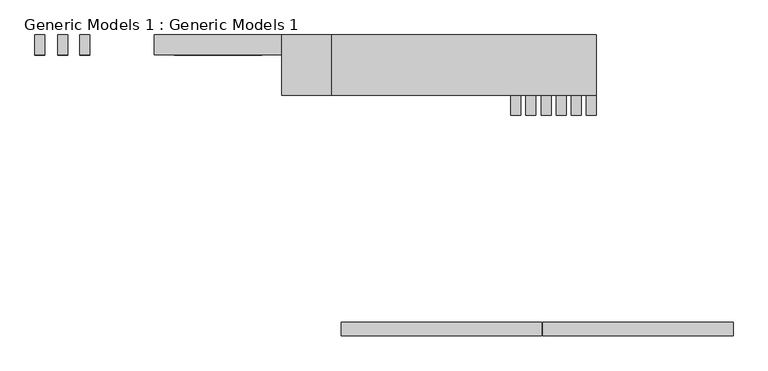
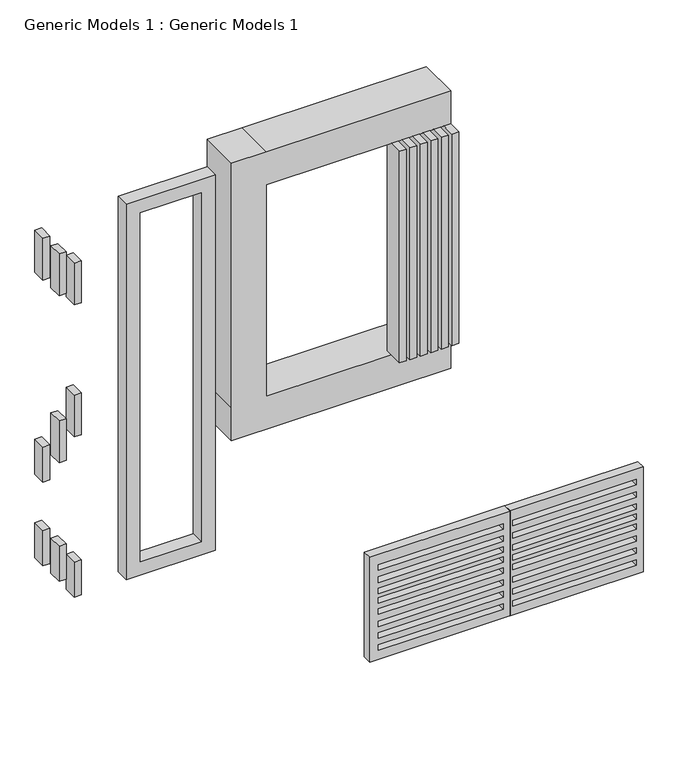
"""IFC4 building model written with IfcOpenShell, lengths in millimetres: proxy geometry, Generic Models 1 : Generic Models 1."""

from ifc_helpers import new_model, si_unit, frame, origin, place, context, project, spatial, polyline, outline, extrude, source, transform, mapped, element, save


def generic_models_1_generic_models_1_2996b52b(model_context):
    return source(origin(), model_context, "Body", "SweptSolid", [
        extrude(outline(polyline([(2263.7323709, 2503.9584916), (-152.4, 2503.9584916), (-152.4, 5399.5584916), (2263.7323709, 5399.5584916), (2263.7323709, 2503.9584916)]), holes=[polyline([(1900.2353757, 2559.0491365), (2027.2353757, 2559.0491365), (2027.2353757, 5251.4491365), (1900.2353757, 5251.4491365), (1900.2353757, 2559.0491365)]), polyline([(1620.8353757, 2559.0491365), (1747.8353757, 2559.0491365), (1747.8353757, 5251.4491365), (1620.8353757, 5251.4491365), (1620.8353757, 2559.0491365)]), polyline([(1341.4353757, 2559.0491365), (1468.4353757, 2559.0491365), (1468.4353757, 5251.4491365), (1341.4353757, 5251.4491365), (1341.4353757, 2559.0491365)]), polyline([(1112.8353757, 2559.0491365), (1239.8353757, 2559.0491365), (1239.8353757, 5251.4491365), (1112.8353757, 5251.4491365), (1112.8353757, 2559.0491365)]), polyline([(884.2353757, 2559.0491365), (1011.2353757, 2559.0491365), (1011.2353757, 5251.4491365), (884.2353757, 5251.4491365), (884.2353757, 2559.0491365)]), polyline([(604.8353757, 2559.0491365), (731.8353757, 2559.0491365), (731.8353757, 5251.4491365), (604.8353757, 5251.4491365), (604.8353757, 2559.0491365)]), polyline([(325.4353757, 2559.0491365), (452.4353757, 2559.0491365), (452.4353757, 5251.4491365), (325.4353757, 5251.4491365), (325.4353757, 2559.0491365)]), polyline([(46.0353757, 2559.0491365), (173.0353757, 2559.0491365), (173.0353757, 5251.4491365), (46.0353757, 5251.4491365), (46.0353757, 2559.0491365)])]), frame((0.0, -10129.8064015, 0.0), z_axis=(0.0, 1.0, 0.0), x_axis=(0.0, 0.0, 1.0)), (0.0, 0.0, 1.0), 203.2),
        extrude(outline(polyline([(-152.4, 2491.2584916), (2263.7323709, 2491.2584916), (2263.7323709, -556.7415084), (-152.4, -556.7415084), (-152.4, 2491.2584916)]), holes=[polyline([(1900.2353757, -369.7660375), (2027.2353757, -369.7660375), (2027.2353757, 2348.0339625), (1900.2353757, 2348.0339625), (1900.2353757, -369.7660375)]), polyline([(1620.8353757, -369.7660375), (1747.8353757, -369.7660375), (1747.8353757, 2348.0339625), (1620.8353757, 2348.0339625), (1620.8353757, -369.7660375)]), polyline([(1366.8353757, -369.7660375), (1493.8353757, -369.7660375), (1493.8353757, 2348.0339625), (1366.8353757, 2348.0339625), (1366.8353757, -369.7660375)]), polyline([(1138.2353757, -369.7660375), (1265.2353757, -369.7660375), (1265.2353757, 2348.0339625), (1138.2353757, 2348.0339625), (1138.2353757, -369.7660375)]), polyline([(884.2353757, -369.7660375), (1011.2353757, -369.7660375), (1011.2353757, 2348.0339625), (884.2353757, 2348.0339625), (884.2353757, -369.7660375)]), polyline([(604.8353757, -369.7660375), (731.8353757, -369.7660375), (731.8353757, 2348.0339625), (604.8353757, 2348.0339625), (604.8353757, -369.7660375)]), polyline([(335.2131579, -369.7660375), (462.2131579, -369.7660375), (462.2131579, 2348.0339625), (335.2131579, 2348.0339625), (335.2131579, -369.7660375)]), polyline([(55.8131579, -369.7660375), (182.8131579, -369.7660375), (182.8131579, 2348.0339625), (55.8131579, 2348.0339625), (55.8131579, -369.7660375)])]), frame((0.0, -10129.8064015, 0.0), z_axis=(0.0, 1.0, 0.0), x_axis=(0.0, 0.0, 1.0)), (0.0, 0.0, 1.0), 203.2),
        extrude(outline(polyline([(-5065.2415084, -5862.6064015), (-5217.6415084, -5862.6064015), (-5217.6415084, -5557.8064015), (-5065.2415084, -5557.8064015), (-5065.2415084, -5862.6064015)])), frame((0.0, 0.0, 7700.2105263), z_axis=(0.0, 0.0, 1.0), x_axis=(1.0, 0.0, 0.0)), (0.0, 0.0, 1.0), 962.5263158),
        extrude(outline(polyline([(-4715.583357, -5862.6064015), (-4867.983357, -5862.6064015), (-4867.983357, -5557.8064015), (-4715.583357, -5557.8064015), (-4715.583357, -5862.6064015)])), frame((0.0, 0.0, 7218.9473684), z_axis=(0.0, 0.0, 1.0), x_axis=(1.0, 0.0, 0.0)), (0.0, 0.0, 1.0), 962.5263158),
        extrude(outline(polyline([(-4386.7201991, -5862.6064015), (-4539.1201991, -5862.6064015), (-4539.1201991, -5557.8064015), (-4386.7201991, -5557.8064015), (-4386.7201991, -5862.6064015)])), frame((0.0, 0.0, 6890.0842105), z_axis=(0.0, 0.0, 1.0), x_axis=(1.0, 0.0, 0.0)), (0.0, 0.0, 1.0), 962.5263158),
        extrude(outline(polyline([(-5065.2415084, -5862.6064015), (-5217.6415084, -5862.6064015), (-5217.6415084, -5557.8064015), (-5065.2415084, -5557.8064015), (-5065.2415084, -5862.6064015)])), frame((0.0, 0.0, 3039.9789474), z_axis=(0.0, 0.0, 1.0), x_axis=(1.0, 0.0, 0.0)), (0.0, 0.0, 1.0), 810.1263158),
        extrude(outline(polyline([(-4715.583357, -5862.6064015), (-4867.983357, -5862.6064015), (-4867.983357, -5557.8064015), (-4715.583357, -5557.8064015), (-4715.583357, -5862.6064015)])), frame((0.0, 0.0, 3368.8421053), z_axis=(0.0, 0.0, 1.0), x_axis=(1.0, 0.0, 0.0)), (0.0, 0.0, 1.0), 962.5263158),
        extrude(outline(polyline([(-4386.7201991, -5862.6064015), (-4539.1201991, -5862.6064015), (-4539.1201991, -5557.8064015), (-4386.7201991, -5557.8064015), (-4386.7201991, -5862.6064015)])), frame((0.0, 0.0, 3850.1052632), z_axis=(0.0, 0.0, 1.0), x_axis=(1.0, 0.0, 0.0)), (0.0, 0.0, 1.0), 962.5263158),
        extrude(outline(polyline([(-5065.2415084, -5862.6064015), (-5217.6415084, -5862.6064015), (-5217.6415084, -5557.8064015), (-5065.2415084, -5557.8064015), (-5065.2415084, -5862.6064015)])), frame((0.0, 0.0, 1114.9263158), z_axis=(0.0, 0.0, 1.0), x_axis=(1.0, 0.0, 0.0)), (0.0, 0.0, 1.0), 810.1263158),
        extrude(outline(polyline([(-4715.583357, -5862.6064015), (-4867.983357, -5862.6064015), (-4867.983357, -5557.8064015), (-4715.583357, -5557.8064015), (-4715.583357, -5862.6064015)])), frame((0.0, 0.0, 633.6631579), z_axis=(0.0, 0.0, 1.0), x_axis=(1.0, 0.0, 0.0)), (0.0, 0.0, 1.0), 810.1263158),
        extrude(outline(polyline([(-4386.7201991, -5862.6064015), (-4539.1201991, -5862.6064015), (-4539.1201991, -5557.8064015), (-4386.7201991, -5557.8064015), (-4386.7201991, -5862.6064015)])), frame((0.0, 0.0, 152.4), z_axis=(0.0, 0.0, 1.0), x_axis=(1.0, 0.0, 0.0)), (0.0, 0.0, 1.0), 810.1263158),
        extrude(outline(polyline([(3316.7584916, -6777.0064015), (3164.3584916, -6777.0064015), (3164.3584916, -6319.8064015), (3316.7584916, -6319.8064015), (3316.7584916, -6777.0064015)])), frame((0.0, 0.0, 3810.0), z_axis=(0.0, 0.0, 1.0), x_axis=(1.0, 0.0, 0.0)), (0.0, 0.0, 1.0), 4876.8),
        extrude(outline(polyline([(3088.1584916, -6777.0064015), (2935.7584916, -6777.0064015), (2935.7584916, -6319.8064015), (3088.1584916, -6319.8064015), (3088.1584916, -6777.0064015)])), frame((0.0, 0.0, 3810.0), z_axis=(0.0, 0.0, 1.0), x_axis=(1.0, 0.0, 0.0)), (0.0, 0.0, 1.0), 4876.8),
        extrude(outline(polyline([(2859.5584916, -6777.0064015), (2707.1584916, -6777.0064015), (2707.1584916, -6319.8064015), (2859.5584916, -6319.8064015), (2859.5584916, -6777.0064015)])), frame((0.0, 0.0, 3810.0), z_axis=(0.0, 0.0, 1.0), x_axis=(1.0, 0.0, 0.0)), (0.0, 0.0, 1.0), 4876.8),
        extrude(outline(polyline([(2630.9584916, -6777.0064015), (2478.5584916, -6777.0064015), (2478.5584916, -6319.8064015), (2630.9584916, -6319.8064015), (2630.9584916, -6777.0064015)])), frame((0.0, 0.0, 3810.0), z_axis=(0.0, 0.0, 1.0), x_axis=(1.0, 0.0, 0.0)), (0.0, 0.0, 1.0), 4876.8),
        extrude(outline(polyline([(2402.3584916, -6777.0064015), (2249.9584916, -6777.0064015), (2249.9584916, -6319.8064015), (2402.3584916, -6319.8064015), (2402.3584916, -6777.0064015)])), frame((0.0, 0.0, 3810.0), z_axis=(0.0, 0.0, 1.0), x_axis=(1.0, 0.0, 0.0)), (0.0, 0.0, 1.0), 4876.8),
        extrude(outline(polyline([(2173.7584916, -6777.0064015), (2021.3584916, -6777.0064015), (2021.3584916, -6319.8064015), (2173.7584916, -6319.8064015), (2173.7584916, -6777.0064015)])), frame((0.0, 0.0, 3810.0), z_axis=(0.0, 0.0, 1.0), x_axis=(1.0, 0.0, 0.0)), (0.0, 0.0, 1.0), 4876.8),
        extrude(outline(polyline([(3048.0, -1461.8220223), (3048.0, 3316.7584916), (3810.0, 3316.7584916), (3810.0, -702.7915084), (8686.8, -702.7915084), (8686.8, 3316.7584916), (9448.8, 3316.7584916), (9448.8, -702.7915084), (9448.8, -1461.8220223), (3810.0, -1461.8220223), (3048.0, -1461.8220223)])), frame((0.0, -6472.2064015, 0.0), z_axis=(0.0, 1.0, 0.0), x_axis=(0.0, 0.0, 1.0)), (0.0, 0.0, 1.0), 914.4),
        extrude(outline(polyline([(157.4131579, -3404.9220223), (157.4131579, -1461.8220223), (8815.1368421, -1461.8220223), (8815.1368421, -3404.9220223), (157.4131579, -3404.9220223)]), holes=[polyline([(8510.3368421, -1766.6220223), (462.2131579, -1766.6220223), (462.2131579, -3100.1220223), (8510.3368421, -3100.1220223), (8510.3368421, -1766.6220223)])]), frame((0.0, -5862.6064015, 0.0), z_axis=(0.0, 1.0, 0.0), x_axis=(0.0, 0.0, 1.0)), (0.0, 0.0, 1.0), 304.8),
    ])


if __name__ == "__main__":
    model = new_model("IFC4")
    model_context = context("Model", 3, world=origin())
    ifc_project = project(units=[si_unit("LENGTHUNIT", "METRE", prefix="MILLI")], contexts=[model_context])
    site = spatial("IfcSite", under=ifc_project)
    building = spatial("IfcBuilding", under=site)
    placement = place(None, origin())
    generic_models_1_generic_models_1_shape = generic_models_1_generic_models_1_2996b52b(model_context)
    element("IfcBuildingElementProxy", 1, Name="Generic Models 1 : Generic Models 1", ObjectType="Generic Models 1 : Generic Models 1", at=placement, inside=building, context=model_context, shape_type="MappedRepresentation", body=[
        mapped(generic_models_1_generic_models_1_shape, transform((0.0, 0.0, 0.0), x_axis=(1.0, 0.0, 0.0), y_axis=(0.0, 1.0, 0.0), z_axis=(0.0, 0.0, 1.0))),
    ])
    save(model, "model.ifc")

# Revit data of these elements
# Element 1 (IfcBuildingElementProxy, "Generic Models 1 : Generic Models 1")
#   Materials on its faces: "wall 1", "Copper", "Wood Planks", "wall"
# Materials
#   "wall 1": class "Generic", colour RGB 67 39 34, transparency 0, Cost = 0
#   "Copper": class "Metal", colour RGB 0 0 0, transparency 0, Description = "Copper, matte finish", Cost = 0
#   "Wood Planks": class "Wood", colour RGB 193 160 115, transparency 0, Description = "Physical material.", Cost = 0
#   "wall": class "Generic", colour RGB 86 92 74, transparency 0, Cost = 0
